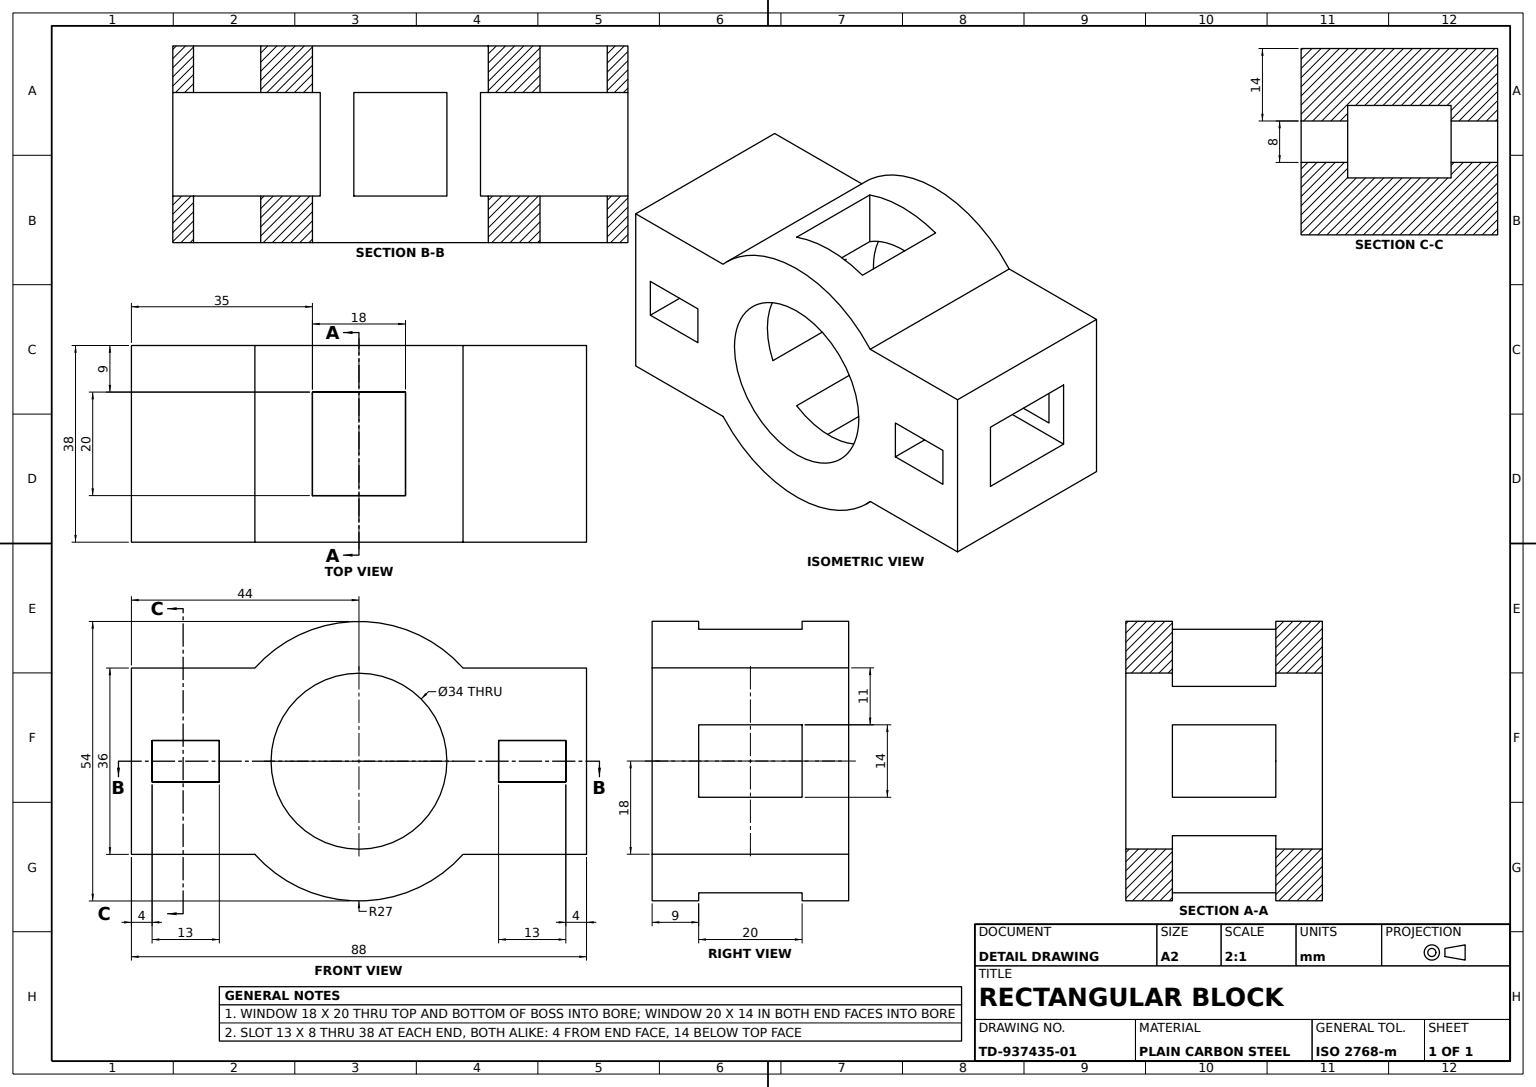
SolidWorks part; units mm, degrees
material "Plain Carbon Steel"
ref_plane "Front Plane" through (0, 0, 0) normal (0, 0, 1) x (1, 0, 0)
ref_plane "Top Plane" through (0, 0, 0) normal (0, 1, 0) x (1, 0, 0)
ref_plane "Right Plane" through (0, 0, 0) normal (1, 0, 0) x (0, 0, -1)
sketch "Body Profile Sketch" plane through (0, 0, 0) normal (0, 0, 1) x (1, 0, 0)
  line L0 (0, 0) -> (0, -17) construction
  line L1 (-44, -18) -> (-20.1246, -18)
  line L2 (-44, -18) -> (-44, 18)
  line L3 (-44, 18) -> (-20.1246, 18)
  line L4 (44, -18) -> (44, 18)
  line L5 (-40, -4) -> (-27, -4)
  line L6 (-40, -4) -> (-40, 4)
  line L7 (20.1246, 18) -> (44, 18)
  line L8 (-40, 4) -> (-27, 4)
  line L9 (20.1246, -18) -> (44, -18)
  line L10 (-27, -4) -> (-27, 4)
  line L15 (40, -4) -> (40, 4)
  line L16 (40, 4) -> (27, 4)
  line L17 (27, -4) -> (27, 4)
  line L18 (40, -4) -> (27, -4)
  arc A0 (-20.1246, -18) -> (20.1246, -18) centre (0, 0) ccw
  arc A1 (20.1246, 18) -> (-20.1246, 18) centre (0, 0) ccw
  circle A2 centre (0, 0) radius 17
  point P0 (0, 0)
  dimension "D3" = 54
  dimension "D4" = 34
  dimension "D1" = 88
  dimension "D2" = 36
  dimension "D5" = 13
  dimension "D6" = 8
  dimension "D7" = 14
  dimension "D8" = 4
  dimension "D9" = 44
  dimension "D10" = 18
extrude "Body Extrude 38mm" add sketch "Body Profile Sketch" against normal blind 38
sketch "Window 18x20 Sketch" plane through (0, 18, 0) normal (0, 1, 0) x (1, 0, 0)
  line L0 (44, 38) -> (20.1246, 38) construction
  line L1 (-9, 9) -> (9, 9)
  line L2 (-9, 9) -> (-9, 29)
  line L3 (-9, 29) -> (9, 29)
  line L4 (9, 9) -> (9, 29)
  line L5 (44, 38) -> (44, 0) construction
  point P4 (0, 29)
  point P7 (9, 19)
  dimension "D1" = 18
  dimension "D2" = 20
  dimension "D3" = 44
  dimension "D4" = 19
sketch "Window 20x14 Sketch" plane through (-44, 0, 0) normal (-1, 0, 0) x (0, 0, 1)
  line L0 (-38, -18) -> (0, -18) construction
  line L1 (-29, -7) -> (-9, -7)
  line L2 (-29, -7) -> (-29, 7)
  line L3 (-29, 7) -> (-9, 7)
  line L4 (-9, -7) -> (-9, 7)
  line L5 (-38, 18) -> (-38, -18) construction
  point P8 (-19, -7)
  dimension "D1" = 20
  dimension "D2" = 14
  dimension "D3" = 25
  dimension "D4" = 19
extrude "Window Cut 20x14" cut sketch "Window 20x14 Sketch" against normal through all both and the other way through all
extrude "Window Cut 18x20" cut sketch "Window 18x20 Sketch" along normal through all and the other way through all
